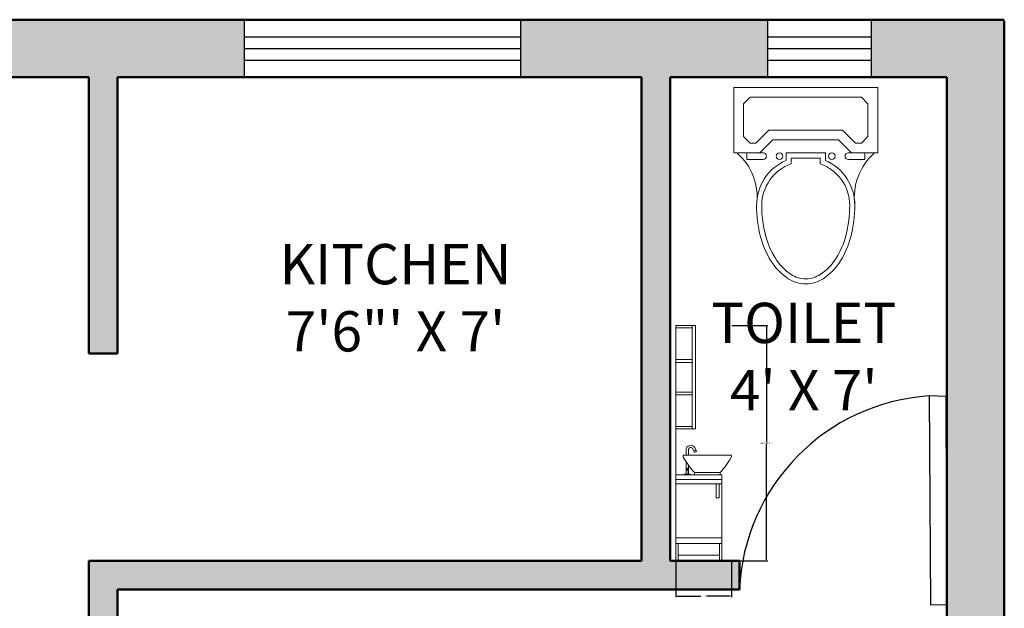
# Model space of a CAD drawing. Units: inches. Extents: x 1771 to 3025, y 319 to 889.
# Tile 24 of 35: x 2390 to 2561, y 786 to 889. Entities that reach past the tile are written whole.
import ezdxf

# ---------------------------------------------------------------- set-up
doc = ezdxf.new("R2010")
doc.units = ezdxf.units.IN
doc.header["$MEASUREMENT"] = 0
for name, color, linetype, lineweight in [('A-ANNO-DIMS', 2, 'Continuous', 18), ('A-AREA-IDEN', 241, 'Continuous', 25), ('A-DOOR', 4, 'Continuous', 25), ('A-FLOR-FIXT', 8, 'Continuous', 18), ('A-GLAZ', 40, 'Continuous', 25), ('A-WALL', 7, 'Continuous', 50), ('A-WALL-PATT', 254, 'Continuous', 13)]:
    doc.layers.add(name, color=color, linetype=linetype, lineweight=lineweight)
doc.styles.get("Standard").update_dxf_attribs({"font": 'arial.ttf'})
doc.dimstyles.get("Standard").update_dxf_attribs({"dimtxt": 0.18, "dimasz": 0.18, "dimexe": 0.18, "dimexo": 0.0625, "dimgap": 0.09, "dimtad": 0, "dimtih": 1, "dimtoh": 1, "dimdec": 4, "dimzin": 0, "dimdsep": 46, "dimtxsty": 'Standard', "dimcen": 0.09, "dimadec": 0, "dimazin": 0, "dimtfac": 1, "dimtdec": 4, "dimtofl": 0, "dimtmove": 0, "dimatfit": 3, "dimfxl": 1, "dimtolj": 1, "dimtzin": 0, "dimarcsym": 0})

# ---------------------------------------------------------------- blocks, each defined once
blk = doc.blocks.new('A$C098B081F')
for p, q in [((558.8, 762), (0, 762)), ((0, 762), (0, 508)), ((558.8, 762), (558.8, 508)), ((63.5, 723.9), (38.1, 698.5)), ((38.1, 698.5), (38.1, 571.5)), ((495.3, 723.9), (63.5, 723.9)), ((520.7, 698.5), (495.3, 723.9)), ((520.7, 698.5), (520.7, 571.5)), ((136.6, 596.9), (85.8, 546.1)), ((422.2, 596.9), (136.6, 596.9)), ((422.2, 596.9), (473, 546.1)), ((38.1, 571.5), (63.5, 546.1)), ((63.5, 546.1), (85.8, 546.1)), ((152.4, 558.8), (101.6, 508)), ((406.4, 558.8), (152.4, 558.8)), ((406.4, 558.8), (457.2, 508)), ((495.3, 546.1), (473, 546.1)), ((495.3, 546.1), (520.7, 571.5)), ((0, 508), (12.7, 508)), ((12.7, 508), (101.6, 508)), ((50.8, 508), (50.8, 482.6)), ((50.8, 508), (101.6, 508)), ((114.3, 508), (101.6, 508)), ((203.2, 508), (203.2, 479.4)), ((203.2, 508), (355.6, 508)), ((355.6, 508), (355.6, 479.4)), ((444.5, 508), (457.2, 508)), ((508, 508), (457.2, 508)), ((508, 508), (546.1, 508)), ((508, 508), (508, 482.6)), ((558.8, 508), (546.1, 508)), ((50.8, 482.6), (114.3, 482.6)), ((223.2, 488), (223.2, 465.8)), ((223.2, 488), (335.6, 488)), ((335.6, 488), (335.6, 465.8)), ((508, 482.6), (444.5, 482.6))]:
    blk.add_line(p, q)
for centre in [(177.8, 495.3), (381, 495.3)]:
    blk.add_circle(centre, 12.7)
for centre, radius, start, end in [((-137.5, 335.8), 228.5, 352.2011, 48.911), ((114.3, 495.3), 12.7, 270, 90), ((444.5, 495.3), 12.7, 90, 270), ((696.3, 335.8), 228.5, 131.089, 187.7989), ((279.4, 304.8), 190.5, 113.5782, 180), ((279.4, 304.8), 170.5, 109.2456, 180), ((279.4, 304.8), 170.5, 0, 70.7544), ((279.4, 304.8), 190.5, 0, 66.4218), ((574.9, 304.8), 486, 180, 194.5143), ((574.9, 304.8), 466, 180, 194.5143), ((-16.1, 304.8), 466, 345.4857, 360), ((-16.1, 304.8), 486, 345.4857, 360), ((429.2, 267.1), 335.5, 194.5143, 212.0054), ((429.2, 267.1), 315.5, 194.5143, 212.0054), ((129.6, 267.1), 315.5, 327.9946, 345.4857), ((129.6, 267.1), 335.5, 327.9946, 345.4857), ((337.2, 209.6), 227, 212.0054, 236.4659), ((337.2, 209.6), 207, 212.0054, 236.4659), ((221.6, 209.6), 207, 303.5341, 327.9946), ((221.6, 209.6), 227, 303.5341, 327.9946), ((279.4, 122.4), 122.4, 236.4659, 270), ((279.4, 122.4), 102.4, 236.4659, 270), ((279.4, 122.4), 102.4, 270, 303.5341), ((279.4, 122.4), 122.4, 270, 303.5341)]:
    blk.add_arc(centre, radius, start, end)
blk = doc.blocks.new('A$C3EAC730C')
for p, q in [((0, 2.05), (0.17, 2.05)), ((0, 2.05), (0, 0.2)), ((0, 2.03), (0.14, 2.03)), ((0.14, 2.05), (0.14, 1.15)), ((0.17, 2.05), (0.17, 1.15)), ((0, 1.7542), (0.14, 1.7542)), ((0, 1.7292), (0.14, 1.7292)), ((0, 1.4708), (0.14, 1.4708)), ((0, 1.4458), (0.14, 1.4458)), ((0, 1.17), (0.14, 1.17)), ((0, 1.15), (0.17, 1.15)), ((0.0877, 0.964), (0.0877, 0.92)), ((0.1077, 0.9647), (0.1077, 0.92)), ((0.1601, 0.9446), (0.1481, 0.9744)), ((0.1545, 0.9582), (0.1731, 0.9657)), ((0.1552, 0.9563), (0.1739, 0.9639)), ((0.1601, 0.9446), (0.1787, 0.9521)), ((0.1787, 0.9521), (0.1666, 0.9819)), ((0.0627, 0.915), (0.0627, 0.9063)), ((0.0677, 0.92), (0.4777, 0.92)), ((0.0877, 0.8637), (0.0877, 0.756)), ((0.4827, 0.915), (0.4827, 0.9063)), ((0.4827, 0.915), (0.4827, 0.9063)), ((0.0902, 0.7905), (0.1052, 0.7905)), ((0.0902, 0.7905), (0.0902, 0.756)), ((0.0947, 0.8022), (0.0947, 0.7905)), ((0.1007, 0.8022), (0.1007, 0.7905)), ((0.1052, 0.7905), (0.1052, 0.756)), ((0.1077, 0.8346), (0.1077, 0.756)), ((0.4, 0.75), (0, 0.75)), ((0.4, 0.71), (0, 0.71)), ((0.0577, 0.75), (0.1037, 0.75)), ((0.0727, 0.756), (0.0727, 0.75)), ((0.1227, 0.756), (0.0727, 0.756)), ((0.1227, 0.756), (0.1227, 0.75)), ((0.1602, 0.77), (0.1602, 0.75)), ((0.1602, 0.77), (0.3852, 0.77)), ((0.1602, 0.75), (0.3852, 0.75)), ((0.3852, 0.77), (0.3852, 0.75)), ((0.4, 0.71), (0.4, 0.75)), ((0.4, 0.72), (0.4, 0.2)), ((0.4, 0.67), (0, 0.67)), ((0.35, 0.55), (0.35, 0.67)), ((0.375, 0.55), (0.375, 0.67)), ((0.35, 0.55), (0.375, 0.55)), ((0.4, 0.2), (0, 0.2)), ((0, 0.2), (0, 0)), ((0.4, 0), (0.4, 0.2)), ((0.4, 0.15), (0, 0.15)), ((0.02, 0.15), (0.02, 0)), ((0.38, 0), (0.38, 0.15)), ((0, 0), (0.4, 0)), ((0.02, 0.05), (0.38, 0.05))]:
    blk.add_line(p, q)
blk.add_circle((0.0977, 0.804), 0.0035)
for centre, radius, start, end in [((0.1286, 0.9665), 0.041, 22.01327, 183.41193), ((0.1286, 0.9665), 0.021, 22.01327, 184.76808), ((0.0677, 0.915), 0.005, 90, 180), ((0.0677, 0.9063), 0.005, 180, 209.45502), ((0.7052, 1.2664), 0.7372, 209.45502, 222.32259), ((-0.1599, 1.2664), 0.7372, 317.67741, 330.54498), ((0.4777, 0.915), 0.005, 0, 90), ((0.4777, 0.9063), 0.005, 330.54498, 0)]:
    blk.add_arc(centre, radius, start, end)
blk = doc.blocks.new('DOOR-35')
blk.add_lwpolyline([(35.88, 36.19), (32.96, 36.3), (33.16, 0), (36, 0.05)], close=True)
blk.add_arc((35.23, 1.11), 35.26, 93.6879, 177.4925)
blk = doc.blocks.new('WIN-48')
for p, q in [((0, 0), (0, 10)), ((48, 0), (48, 10)), ((0, 7), (48, 7)), ((0, 5), (48, 5)), ((0, 3), (48, 3))]:
    blk.add_line(p, q)
blk = doc.blocks.new('WIN-18')
for p, q in [((0, 0), (0, 10)), ((18, 0), (18, 10)), ((0, 7), (18, 7)), ((0, 5), (18, 5)), ((0, 3), (18, 3))]:
    blk.add_line(p, q)
blk = doc.blocks.new('*D58')
at = {"layer": 'A-ANNO-DIMS', "color": 0, "lineweight": -2, "transparency": 16777216}
for p, q in [((2513.82, 835.5), (2520.07, 835.5)), ((2519.89, 835.32), (2519.89, 815.25)), ((2519.89, 794.81), (2519.89, 814.88)), ((2513.82, 794.63), (2520.07, 794.63))]:
    blk.add_line(p, q, dxfattribs=at)
at = {"layer": 'A-ANNO-DIMS', "color": 0, "transparency": 16777216}
for points in [[(2519.86, 835.32), (2519.92, 835.32), (2519.89, 835.5)], [(2519.86, 794.81), (2519.92, 794.81), (2519.89, 794.63)]]:
    blk.add_solid(points, dxfattribs=at)
at = {"layer": 'Defpoints', "color": 0, "transparency": 16777216}
for p in [(2513.76, 835.5), (2519.89, 835.5), (2513.76, 794.63)]:
    blk.add_point(p, dxfattribs=at)
at = {"layer": 'A-ANNO-DIMS', "color": 0, "transparency": 16777216, "insert": (2519.89, 815.07), "char_height": 0.18, "attachment_point": 5}
blk.add_mtext('\\A1;VANITY UNIT 41 TYP.', dxfattribs=at)
blk = doc.blocks.new('*D59')
at = {"layer": 'A-ANNO-DIMS', "color": 0, "lineweight": -2, "transparency": 16777216}
for p, q in [((2504.14, 794.57), (2504.14, 788.32)), ((2513.76, 794.57), (2513.76, 788.32)), ((2504.32, 788.5), (2508.43, 788.5)), ((2513.58, 788.5), (2509.47, 788.5))]:
    blk.add_line(p, q, dxfattribs=at)
at = {"layer": 'A-ANNO-DIMS', "color": 0, "transparency": 16777216}
for points in [[(2504.32, 788.53), (2504.32, 788.47), (2504.14, 788.5)], [(2513.58, 788.53), (2513.58, 788.47), (2513.76, 788.5)]]:
    blk.add_solid(points, dxfattribs=at)
at = {"layer": 'Defpoints', "color": 0, "transparency": 16777216}
for p in [(2504.14, 794.63), (2513.76, 794.63), (2513.76, 788.5)]:
    blk.add_point(p, dxfattribs=at)
at = {"layer": 'A-ANNO-DIMS', "color": 0, "transparency": 16777216, "insert": (2508.95, 788.5), "char_height": 0.18, "attachment_point": 5}
blk.add_mtext('\\A1;10 TYP.', dxfattribs=at)

msp = doc.modelspace()

# ---------------------------------------------------------------- hatches: boundary and pattern name
at = {"layer": 'A-WALL-PATT'}
h = msp.add_hatch(color=256, dxfattribs=at)
h.dxf.hatch_style = 1
h.paths.add_polyline_path([(2407.16, 878.63), (2429.21, 878.63), (2429.21, 888.63), (2379.16, 888.63), (2379.16, 878.63), (2402.16, 878.63), (2402.16, 830.63), (2407.16, 830.63)])
h.paths.add_polyline_path([(2520.11, 888.63), (2477.21, 888.63), (2477.21, 878.63), (2498.16, 878.63), (2498.16, 794.63), (2402.16, 794.63), (2402.16, 758.63), (2402.16, 664.63), (2407.16, 664.63), (2407.16, 712), (2407.16, 789.63), (2515.16, 789.63), (2515.16, 794.63), (2503.16, 794.63), (2503.16, 878.63), (2520.11, 878.63)])
h.paths.add_polyline_path([(2561.16, 888.63), (2538.11, 888.63), (2538.11, 878.63), (2551.16, 878.63), (2551.16, 789.63), (2551.16, 768.61), (2561.16, 768.61)])
h.paths.add_polyline_path([(2561.16, 720.61), (2551.16, 720.61), (2551.16, 669.63), (2443.16, 669.63), (2443.16, 664.63), (2462.16, 664.63), (2462.16, 652.63), (2467.16, 652.63), (2467.16, 664.63), (2551.16, 664.63), (2551.16, 649.17), (2561.16, 649.17)])
h.paths.add_polyline_path([(2561.16, 631.17), (2551.16, 631.17), (2551.16, 616.63), (2462.16, 616.63), (2443.16, 616.63), (2443.16, 611.63), (2551.16, 611.63), (2551.16, 581.11), (2561.16, 581.11)])
h.paths.add_polyline_path([(2561.16, 533.11), (2551.16, 533.11), (2551.16, 479.63), (2407.16, 479.63), (2407.16, 616.63), (2397.16, 616.63), (2397.16, 543.63), (2306.16, 543.63), (2306.16, 533.63), (2397.16, 533.63), (2397.16, 469.63), (2551.16, 469.63), (2551.16, 452.76), (2561.16, 452.76)])
h.paths.add_polyline_path([(2561.16, 404.76), (2551.16, 404.76), (2551.16, 393.63), (2397.16, 393.63), (2397.16, 383.63), (2561.16, 383.63)])
h.paths.add_polyline_path([(2270.16, 642.58), (2260.16, 642.58), (2260.16, 533.63), (2270.16, 533.63)])
h.paths.add_polyline_path([(2270.16, 753.63), (2366.16, 753.63), (2366.16, 758.63), (2270.16, 758.63), (2270.16, 842.59, -0.008336), (2268.86, 842.63), (2260.16, 842.63), (2260.16, 690.58), (2270.16, 690.58)])
h.paths.add_polyline_path([(2331.16, 888.63), (2260.16, 888.63), (2260.16, 878.63), (2331.16, 878.63)])

# ---------------------------------------------------------------- linework, layer by layer
at = {"layer": 'A-WALL'}
for p, q in [((2561.16, 888.63), (2219.16, 888.63)), ((2561.16, 383.63), (2561.16, 888.43)), ((2402.16, 878.63), (2224.16, 878.63)), ((2402.16, 878.63), (2402.16, 830.63)), ((2498.16, 878.63), (2407.16, 878.63)), ((2407.16, 878.63), (2407.16, 830.63)), ((2498.16, 794.63), (2498.16, 878.63)), ((2503.16, 794.63), (2503.16, 878.63)), ((2551.16, 878.63), (2503.16, 878.63)), ((2551.16, 789.63), (2551.16, 878.63)), ((2407.16, 830.63), (2402.16, 830.63)), ((2498.16, 794.63), (2402.16, 794.63)), ((2402.16, 794.63), (2402.16, 758.63)), ((2515.16, 794.63), (2503.16, 794.63)), ((2515.16, 789.63), (2515.16, 794.63)), ((2515.16, 789.63), (2407.16, 789.63)), ((2407.16, 789.63), (2407.16, 669.63)), ((2551.16, 669.63), (2551.16, 789.63))]:
    msp.add_line(p, q, dxfattribs=at)

# ---------------------------------------------------------------- block references
at = {"layer": 'A-DOOR'}
msp.add_blockref('DOOR-35', (2515.16, 786.98), dxfattribs=at)
at = {"layer": 'A-FLOR-FIXT'}
for name, p, xscale, yscale, zscale in [('A$C098B081F', (2514.16, 842.73), 0.0447923195545138, 0.0447923195545138, 0.0447923195545138), ('A$C3EAC730C', (2504.14, 794.63), 19.93356852258053, 19.93356852258053, 19.93356852258053)]:
    msp.add_blockref(name, p, dxfattribs=dict(at, xscale=xscale, yscale=yscale, zscale=zscale))
at = {"layer": 'A-GLAZ'}
for name, p in [('WIN-48', (2429.21, 878.63)), ('WIN-18', (2520.11, 878.63))]:
    msp.add_blockref(name, p, dxfattribs=at)

# ---------------------------------------------------------------- texts
at = {"layer": 'A-AREA-IDEN', "char_height": 7, "attachment_point": 1}
for s, insert in [('\\pxqc;KITCHEN\\P7\'6"\' X 7\'', (2412.7, 849.67)), ("\\pxqc;TOILET\\P4' X 7'", (2483.6, 839.46))]:
    msp.add_mtext_dynamic_manual_height_columns(s, width=85.4611, gutter_width=1, heights=[0], dxfattribs=dict(at, insert=insert))

# ---------------------------------------------------------------- dimensions: what is measured, and where the dimension line sits
at = {"layer": 'A-ANNO-DIMS'}
dim = msp.add_linear_dim(base=(2519.89, 835.5), p1=(2513.76, 794.63), p2=(2513.76, 835.5), angle=90, text='VANITY UNIT <> TYP.', dimstyle='Standard', override={"dimdec": 0, "dimrnd": 0, "dimzin": 0, "dimlunit": 2}, dxfattribs=at)
dim.commit()
dim.dimension.update_dxf_attribs({"geometry": '*D58', "text_midpoint": (2519.89, 815.07)})
dim = msp.add_linear_dim(base=(2513.76, 788.5), p1=(2504.14, 794.63), p2=(2513.76, 794.63), text='<> TYP.', dimstyle='Standard', override={"dimdec": 0, "dimrnd": 0, "dimzin": 0, "dimlunit": 2}, dxfattribs=at)
dim.commit()
dim.dimension.update_dxf_attribs({"geometry": '*D59', "text_midpoint": (2508.95, 788.5)})

doc.saveas('drawing.dxf')
